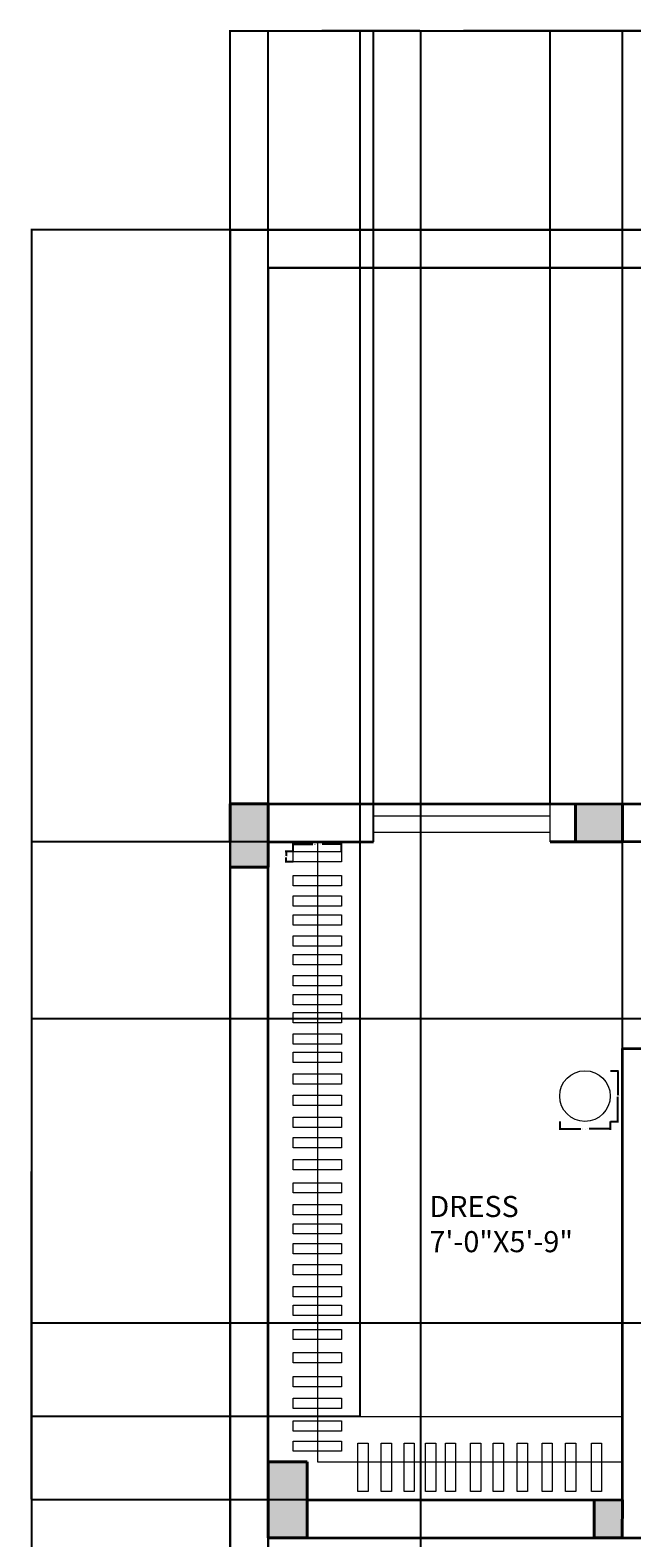
# Model space of a CAD drawing. Units: inches. Extents: x 1210 to 1836, y 84 to 1122.
# Tile 3 of 5: x 1210 to 1353, y 764 to 1122. Entities that reach past the tile are written whole.
import ezdxf

# ---------------------------------------------------------------- set-up
doc = ezdxf.new("R2010")
doc.units = ezdxf.units.IN
doc.header["$MEASUREMENT"] = 0
for name, color, linetype, lineweight in [('A-ANNO-DIMS', 2, 'Continuous', 18), ('A-AREA-IDEN', 7, 'Continuous', 25), ('A-COLS', 7, 'Continuous', 40), ('A-COLS-PATT', 6, 'Continuous', 13), ('A-FURN', 9, 'Continuous', 18), ('A-FURN-FIXD', 32, 'Continuous', 18), ('A-GLAZ', 4, 'Continuous', 18), ('A-WALL', 7, 'Continuous', 35), ('C-PROP', 32, 'Continuous', 30)]:
    doc.layers.add(name, color=color, linetype=linetype, lineweight=lineweight)
doc.styles.get("Standard").update_dxf_attribs({"font": 'arial.ttf'})
doc.dimstyles.get("Standard").update_dxf_attribs({"dimtxt": 0.18, "dimasz": 0.18, "dimexe": 0.18, "dimexo": 0.0625, "dimgap": 0.09, "dimtad": 0, "dimtih": 1, "dimtoh": 1, "dimdec": 4, "dimzin": 0, "dimdsep": 46, "dimtxsty": 'Standard', "dimcen": 0.09, "dimadec": 0, "dimazin": 0, "dimtfac": 1, "dimtdec": 4, "dimtofl": 0, "dimtmove": 0, "dimatfit": 3, "dimfxl": 1, "dimtolj": 1, "dimtzin": 0, "dimarcsym": 0})

# ---------------------------------------------------------------- blocks, each defined once
blk = doc.blocks.new('WARDROBE-HANGER')
for p, q in [((0, 0), (0, 2.42)), ((0, 2.42), (11.47, 2.42)), ((10.31, 0), (0, 0)), ((11.47, 0), (10.31, 0)), ((11.47, 2.42), (11.47, 0))]:
    blk.add_line(p, q)
blk = doc.blocks.new('STOOL-ROUND')
blk.add_circle((6, 6), 6)
blk = doc.blocks.new('*D12')
at = {"layer": 'A-ANNO-DIMS', "color": 0, "lineweight": -2, "transparency": 16777216}
for p, q in [((1272.27, 926.95), (1272.27, 928.79)), ((1272.45, 928.61), (1276.9, 928.61)), ((1283.55, 928.61), (1279.1, 928.61)), ((1283.73, 926.95), (1283.73, 928.79))]:
    blk.add_line(p, q, dxfattribs=at)
at = {"layer": 'A-ANNO-DIMS', "color": 0, "transparency": 16777216}
for points in [[(1272.45, 928.64), (1272.45, 928.58), (1272.27, 928.61)], [(1283.55, 928.64), (1283.55, 928.58), (1283.73, 928.61)]]:
    blk.add_solid(points, dxfattribs=at)
at = {"layer": 'Defpoints', "color": 0, "transparency": 16777216}
for p in [(1272.27, 926.89), (1283.73, 928.61), (1283.73, 926.89)]:
    blk.add_point(p, dxfattribs=at)
at = {"layer": 'A-ANNO-DIMS', "color": 0, "transparency": 16777216, "insert": (1278, 928.61), "char_height": 0.18, "attachment_point": 5}
blk.add_mtext('\\A1;HANGER 11 TYP.', dxfattribs=at)
blk = doc.blocks.new('*D13')
at = {"layer": 'A-ANNO-DIMS', "color": 0, "lineweight": -2, "transparency": 16777216}
for p, q in [((1272.2, 926.89), (1270.37, 926.89)), ((1270.55, 926.71), (1270.55, 925.85)), ((1272.2, 924.46), (1270.37, 924.46)), ((1270.55, 924.64), (1270.55, 925.49))]:
    blk.add_line(p, q, dxfattribs=at)
at = {"layer": 'A-ANNO-DIMS', "color": 0, "transparency": 16777216}
for points in [[(1270.52, 926.71), (1270.58, 926.71), (1270.55, 926.89)], [(1270.52, 924.64), (1270.58, 924.64), (1270.55, 924.46)]]:
    blk.add_solid(points, dxfattribs=at)
at = {"layer": 'Defpoints', "color": 0, "transparency": 16777216}
for p in [(1270.55, 926.89), (1272.27, 926.89), (1272.27, 924.46)]:
    blk.add_point(p, dxfattribs=at)
at = {"layer": 'A-ANNO-DIMS', "color": 0, "transparency": 16777216, "insert": (1270.55, 925.67), "char_height": 0.18, "attachment_point": 5}
blk.add_mtext('\\A1;2 TYP.', dxfattribs=at)
blk = doc.blocks.new('*D14')
at = {"layer": 'A-ANNO-DIMS', "color": 0, "lineweight": -2, "transparency": 16777216}
for p, q in [((1335.45, 862.86), (1335.45, 860.95)), ((1347.45, 862.86), (1347.45, 860.95)), ((1335.63, 861.13), (1340.46, 861.13)), ((1347.27, 861.13), (1342.44, 861.13))]:
    blk.add_line(p, q, dxfattribs=at)
at = {"layer": 'A-ANNO-DIMS', "color": 0, "transparency": 16777216}
for points in [[(1335.63, 861.16), (1335.63, 861.1), (1335.45, 861.13)], [(1347.27, 861.16), (1347.27, 861.1), (1347.45, 861.13)]]:
    blk.add_solid(points, dxfattribs=at)
at = {"layer": 'Defpoints', "color": 0, "transparency": 16777216}
for p in [(1335.45, 862.93), (1347.45, 862.93), (1347.45, 861.13)]:
    blk.add_point(p, dxfattribs=at)
at = {"layer": 'A-ANNO-DIMS', "color": 0, "transparency": 16777216, "insert": (1341.45, 861.13), "char_height": 0.18, "attachment_point": 5}
blk.add_mtext('\\A1;STOOL 12 TYP.', dxfattribs=at)
blk = doc.blocks.new('*D15')
at = {"layer": 'A-ANNO-DIMS', "color": 0, "lineweight": -2, "transparency": 16777216}
for p, q in [((1347.51, 874.92), (1349.43, 874.92)), ((1349.25, 874.74), (1349.25, 869.11)), ((1349.25, 863.11), (1349.25, 868.74)), ((1347.51, 862.93), (1349.43, 862.93))]:
    blk.add_line(p, q, dxfattribs=at)
at = {"layer": 'A-ANNO-DIMS', "color": 0, "transparency": 16777216}
for points in [[(1349.22, 874.74), (1349.28, 874.74), (1349.25, 874.92)], [(1349.22, 863.11), (1349.28, 863.11), (1349.25, 862.93)]]:
    blk.add_solid(points, dxfattribs=at)
at = {"layer": 'Defpoints', "color": 0, "transparency": 16777216}
for p in [(1347.45, 874.92), (1349.25, 874.92), (1347.45, 862.93)]:
    blk.add_point(p, dxfattribs=at)
at = {"layer": 'A-ANNO-DIMS', "color": 0, "transparency": 16777216, "insert": (1349.25, 868.92), "char_height": 0.18, "attachment_point": 5}
blk.add_mtext('\\A1;12 TYP.', dxfattribs=at)
blk = doc.blocks.new('*D22')
at = {"layer": 'A-ANNO-DIMS', "color": 0, "lineweight": -2, "transparency": 16777216}
for p, q in [((1257.32, 1074.28), (1257.32, 1121.57)), ((1257.5, 1121.39), (1522.55, 1121.39)), ((1788.14, 1121.39), (1523.1, 1121.39)), ((1788.32, 1074.28), (1788.32, 1121.57))]:
    blk.add_line(p, q, dxfattribs=at)
at = {"layer": 'A-ANNO-DIMS', "color": 0, "transparency": 16777216}
for points in [[(1257.5, 1121.42), (1257.5, 1121.36), (1257.32, 1121.39)], [(1788.14, 1121.42), (1788.14, 1121.36), (1788.32, 1121.39)]]:
    blk.add_solid(points, dxfattribs=at)
at = {"layer": 'Defpoints', "color": 0, "transparency": 16777216}
for p in [(1788.32, 1121.39), (1257.32, 1074.21), (1788.32, 1074.21)]:
    blk.add_point(p, dxfattribs=at)
at = {"layer": 'A-ANNO-DIMS', "color": 0, "transparency": 16777216, "insert": (1522.82, 1121.39), "char_height": 0.18, "attachment_point": 5}
blk.add_mtext('\\A1;531', dxfattribs=at)
blk = doc.blocks.new('*D23')
at = {"layer": 'A-ANNO-DIMS', "color": 0, "lineweight": -2, "transparency": 16777216}
for p, q in [((1257.26, 1074.21), (1209.97, 1074.21)), ((1210.15, 1074.03), (1210.15, 602.9)), ((1210.15, 131.39), (1210.15, 602.53)), ((1257.26, 131.21), (1209.97, 131.21))]:
    blk.add_line(p, q, dxfattribs=at)
at = {"layer": 'A-ANNO-DIMS', "color": 0, "transparency": 16777216}
for points in [[(1210.12, 1074.03), (1210.18, 1074.03), (1210.15, 1074.21)], [(1210.12, 131.39), (1210.18, 131.39), (1210.15, 131.21)]]:
    blk.add_solid(points, dxfattribs=at)
at = {"layer": 'Defpoints', "color": 0, "transparency": 16777216}
for p in [(1210.15, 1074.21), (1257.32, 1074.21), (1257.32, 131.21)]:
    blk.add_point(p, dxfattribs=at)
at = {"layer": 'A-ANNO-DIMS', "color": 0, "transparency": 16777216, "insert": (1210.15, 602.71), "char_height": 0.18, "attachment_point": 5}
blk.add_mtext('\\A1;943', dxfattribs=at)
blk = doc.blocks.new('*D38')
at = {"layer": 'A-ANNO-DIMS', "color": 0, "lineweight": -2, "transparency": 16777216}
for p, q in [((1266.26, 929.21), (1209.97, 929.21)), ((1210.15, 929.03), (1210.15, 851.4)), ((1210.15, 773.39), (1210.15, 851.03)), ((1266.26, 773.21), (1209.97, 773.21))]:
    blk.add_line(p, q, dxfattribs=at)
at = {"layer": 'A-ANNO-DIMS', "color": 0, "transparency": 16777216}
for points in [[(1210.12, 929.03), (1210.18, 929.03), (1210.15, 929.21)], [(1210.12, 773.39), (1210.18, 773.39), (1210.15, 773.21)]]:
    blk.add_solid(points, dxfattribs=at)
at = {"layer": 'Defpoints', "color": 0, "transparency": 16777216}
for p in [(1210.15, 929.21), (1266.32, 929.21), (1266.32, 773.21)]:
    blk.add_point(p, dxfattribs=at)
at = {"layer": 'A-ANNO-DIMS', "color": 0, "transparency": 16777216, "insert": (1210.15, 851.21), "char_height": 0.18, "attachment_point": 5}
blk.add_mtext('\\A1;156', dxfattribs=at)
blk = doc.blocks.new('*D40')
at = {"layer": 'A-ANNO-DIMS', "color": 0, "lineweight": -2, "transparency": 16777216}
for p, q in [((1288.13, 793.02), (1288.13, 1121.57)), ((1288.31, 1121.39), (1318.9, 1121.39)), ((1350.14, 1121.39), (1319.55, 1121.39)), ((1350.32, 793.02), (1350.32, 1121.57))]:
    blk.add_line(p, q, dxfattribs=at)
at = {"layer": 'A-ANNO-DIMS', "color": 0, "transparency": 16777216}
for points in [[(1288.31, 1121.42), (1288.31, 1121.36), (1288.13, 1121.39)], [(1350.14, 1121.42), (1350.14, 1121.36), (1350.32, 1121.39)]]:
    blk.add_solid(points, dxfattribs=at)
at = {"layer": 'Defpoints', "color": 0, "transparency": 16777216}
for p in [(1350.32, 1121.39), (1288.13, 792.95), (1350.32, 792.95)]:
    blk.add_point(p, dxfattribs=at)
at = {"layer": 'A-ANNO-DIMS', "color": 0, "transparency": 16777216, "insert": (1319.23, 1121.39), "char_height": 0.18, "attachment_point": 5}
blk.add_mtext('\\A1;62.2', dxfattribs=at)
blk = doc.blocks.new('*D41')
at = {"layer": 'A-ANNO-DIMS', "color": 0, "lineweight": -2, "transparency": 16777216}
for p, q in [((1288.07, 792.95), (1209.97, 792.95)), ((1210.15, 792.77), (1210.15, 783.27)), ((1210.15, 773.39), (1210.15, 782.9)), ((1275.46, 773.21), (1209.97, 773.21))]:
    blk.add_line(p, q, dxfattribs=at)
at = {"layer": 'A-ANNO-DIMS', "color": 0, "transparency": 16777216}
for points in [[(1210.12, 792.77), (1210.18, 792.77), (1210.15, 792.95)], [(1210.12, 773.39), (1210.18, 773.39), (1210.15, 773.21)]]:
    blk.add_solid(points, dxfattribs=at)
at = {"layer": 'Defpoints', "color": 0, "transparency": 16777216}
for p in [(1210.15, 792.95), (1288.13, 792.95), (1275.52, 773.21)]:
    blk.add_point(p, dxfattribs=at)
at = {"layer": 'A-ANNO-DIMS', "color": 0, "transparency": 16777216, "insert": (1210.15, 783.08), "char_height": 0.18, "attachment_point": 5}
blk.add_mtext('\\A1;19.74', dxfattribs=at)
blk = doc.blocks.new('*D45')
at = {"layer": 'A-ANNO-DIMS', "color": 0, "lineweight": -2, "transparency": 16777216}
for p, q in [((1449.78, 887.21), (1209.97, 887.21)), ((1210.15, 887.03), (1210.15, 851.34)), ((1210.15, 815.3), (1210.15, 850.98)), ((1449.78, 815.12), (1209.97, 815.12))]:
    blk.add_line(p, q, dxfattribs=at)
at = {"layer": 'A-ANNO-DIMS', "color": 0, "transparency": 16777216}
for points in [[(1210.12, 887.03), (1210.18, 887.03), (1210.15, 887.21)], [(1210.12, 815.3), (1210.18, 815.3), (1210.15, 815.12)]]:
    blk.add_solid(points, dxfattribs=at)
at = {"layer": 'Defpoints', "color": 0, "transparency": 16777216}
for p in [(1449.85, 887.21), (1210.15, 815.12), (1449.85, 815.12)]:
    blk.add_point(p, dxfattribs=at)
at = {"layer": 'A-ANNO-DIMS', "color": 0, "transparency": 16777216, "insert": (1210.15, 851.16), "char_height": 0.18, "attachment_point": 5}
blk.add_mtext('\\A1;72.1', dxfattribs=at)
blk = doc.blocks.new('*D49')
at = {"layer": 'A-ANNO-DIMS', "color": 0, "lineweight": -2, "transparency": 16777216}
for p, q in [((1266.32, 929.28), (1266.32, 1121.57)), ((1266.5, 1121.39), (1278.6, 1121.39)), ((1291.14, 1121.39), (1279.05, 1121.39)), ((1291.32, 929.28), (1291.32, 1121.57))]:
    blk.add_line(p, q, dxfattribs=at)
at = {"layer": 'A-ANNO-DIMS', "color": 0, "transparency": 16777216}
for points in [[(1266.5, 1121.42), (1266.5, 1121.36), (1266.32, 1121.39)], [(1291.14, 1121.42), (1291.14, 1121.36), (1291.32, 1121.39)]]:
    blk.add_solid(points, dxfattribs=at)
at = {"layer": 'Defpoints', "color": 0, "transparency": 16777216}
for p in [(1291.32, 1121.39), (1266.32, 929.21), (1291.32, 929.21)]:
    blk.add_point(p, dxfattribs=at)
at = {"layer": 'A-ANNO-DIMS', "color": 0, "transparency": 16777216, "insert": (1278.82, 1121.39), "char_height": 0.18, "attachment_point": 5}
blk.add_mtext('\\A1;25', dxfattribs=at)
blk = doc.blocks.new('*D50')
at = {"layer": 'A-ANNO-DIMS', "color": 0, "lineweight": -2, "transparency": 16777216}
for p, q in [((1291.32, 938.28), (1291.32, 1121.57)), ((1291.5, 1121.39), (1311.87, 1121.39)), ((1333.03, 1121.39), (1312.66, 1121.39)), ((1333.21, 938.28), (1333.21, 1121.57))]:
    blk.add_line(p, q, dxfattribs=at)
at = {"layer": 'A-ANNO-DIMS', "color": 0, "transparency": 16777216}
for points in [[(1291.5, 1121.42), (1291.5, 1121.36), (1291.32, 1121.39)], [(1333.03, 1121.42), (1333.03, 1121.36), (1333.21, 1121.39)]]:
    blk.add_solid(points, dxfattribs=at)
at = {"layer": 'Defpoints', "color": 0, "transparency": 16777216}
for p in [(1333.21, 1121.39), (1291.32, 938.21), (1333.21, 938.21)]:
    blk.add_point(p, dxfattribs=at)
at = {"layer": 'A-ANNO-DIMS', "color": 0, "transparency": 16777216, "insert": (1312.26, 1121.39), "char_height": 0.18, "attachment_point": 5}
blk.add_mtext('\\A1;41.88', dxfattribs=at)
blk = doc.blocks.new('*D51')
at = {"layer": 'A-ANNO-DIMS', "color": 0, "lineweight": -2, "transparency": 16777216}
for p, q in [((1333.21, 938.28), (1333.21, 1121.57)), ((1333.39, 1121.39), (1364.51, 1121.39)), ((1396.41, 1121.39), (1365.29, 1121.39)), ((1396.59, 938.28), (1396.59, 1121.57))]:
    blk.add_line(p, q, dxfattribs=at)
at = {"layer": 'A-ANNO-DIMS', "color": 0, "transparency": 16777216}
for points in [[(1333.39, 1121.42), (1333.39, 1121.36), (1333.21, 1121.39)], [(1396.41, 1121.42), (1396.41, 1121.36), (1396.59, 1121.39)]]:
    blk.add_solid(points, dxfattribs=at)
at = {"layer": 'Defpoints', "color": 0, "transparency": 16777216}
for p in [(1396.59, 1121.39), (1333.21, 938.21), (1396.59, 938.21)]:
    blk.add_point(p, dxfattribs=at)
at = {"layer": 'A-ANNO-DIMS', "color": 0, "transparency": 16777216, "insert": (1364.9, 1121.39), "char_height": 0.18, "attachment_point": 5}
blk.add_mtext('\\A1;63.39', dxfattribs=at)
blk = doc.blocks.new('*D72')
at = {"layer": 'A-ANNO-DIMS', "color": 0, "lineweight": -2, "transparency": 16777216}
for p, q in [((1257.32, 590.28), (1257.32, 1121.57)), ((1257.5, 1121.39), (1279.44, 1121.39)), ((1302.31, 1121.39), (1280.37, 1121.39)), ((1302.49, 590.28), (1302.49, 1121.57))]:
    blk.add_line(p, q, dxfattribs=at)
at = {"layer": 'A-ANNO-DIMS', "color": 0, "transparency": 16777216}
for points in [[(1257.5, 1121.42), (1257.5, 1121.36), (1257.32, 1121.39)], [(1302.31, 1121.42), (1302.31, 1121.36), (1302.49, 1121.39)]]:
    blk.add_solid(points, dxfattribs=at)
at = {"layer": 'Defpoints', "color": 0, "transparency": 16777216}
for p in [(1302.49, 1121.39), (1257.32, 590.21), (1302.49, 590.21)]:
    blk.add_point(p, dxfattribs=at)
at = {"layer": 'A-ANNO-DIMS', "color": 0, "transparency": 16777216, "insert": (1279.91, 1121.39), "char_height": 0.18, "attachment_point": 5}
blk.add_mtext('\\A1;45.165', dxfattribs=at)
blk = doc.blocks.new('*D73')
at = {"layer": 'A-ANNO-DIMS', "color": 0, "lineweight": -2, "transparency": 16777216}
for p, q in [((1302.49, 590.28), (1302.49, 1121.57)), ((1302.67, 1121.39), (1339.91, 1121.39)), ((1377.81, 1121.39), (1340.56, 1121.39)), ((1377.99, 590.28), (1377.99, 1121.57))]:
    blk.add_line(p, q, dxfattribs=at)
at = {"layer": 'A-ANNO-DIMS', "color": 0, "transparency": 16777216}
for points in [[(1302.67, 1121.42), (1302.67, 1121.36), (1302.49, 1121.39)], [(1377.81, 1121.42), (1377.81, 1121.36), (1377.99, 1121.39)]]:
    blk.add_solid(points, dxfattribs=at)
at = {"layer": 'Defpoints', "color": 0, "transparency": 16777216}
for p in [(1377.99, 1121.39), (1302.49, 590.21), (1377.99, 590.21)]:
    blk.add_point(p, dxfattribs=at)
at = {"layer": 'A-ANNO-DIMS', "color": 0, "transparency": 16777216, "insert": (1340.24, 1121.39), "char_height": 0.18, "attachment_point": 5}
blk.add_mtext('\\A1;75.5', dxfattribs=at)

msp = doc.modelspace()

# ---------------------------------------------------------------- hatches: boundary and pattern name
at = {"layer": 'A-COLS-PATT'}
h = msp.add_hatch(color=256, dxfattribs=at)
h.dxf.hatch_style = 1
h.paths.add_polyline_path([(1266.3239, 938.214), (1257.3239, 938.214), (1257.3239, 929.4573), (1257.3239, 923.2025), (1266.3239, 923.2025)])
h.paths.add_polyline_path([(1350.3239, 929.214), (1350.3239, 938.214), (1339.1886, 938.214), (1339.1886, 929.214)])
h.paths.add_polyline_path([(1559.1961, 929.214), (1559.1961, 938.214), (1542.8626, 938.214), (1542.8626, 929.214), (1543.3239, 929.214)])
h.paths.add_polyline_path([(1771.5139, 938.214), (1771.5139, 929.214), (1788.3239, 929.214), (1788.3239, 938.214)])
h.paths.add_polyline_path([(1788.3239, 764.214), (1788.3239, 773.214), (1775.2119, 773.214), (1775.2119, 764.214)])
h.paths.add_polyline_path([(1552.3239, 764.214), (1552.3239, 773.214), (1543.3239, 773.214), (1535.8494, 773.197), (1535.8494, 764.214)])
h.paths.add_polyline_path([(1275.5217, 782.2138), (1272.7843, 782.2138), (1266.3239, 782.2138), (1266.3239, 764.214), (1275.5217, 764.214)])
h.paths.add_polyline_path([(1350.2372, 764.214), (1350.3239, 773.214), (1343.6352, 773.214), (1343.6352, 764.214)])
h.paths.add_polyline_path([(1257.3239, 570.3846), (1266.3239, 570.3846), (1266.3239, 590.214), (1257.3239, 590.214)])
h.paths.add_polyline_path([(1450.8239, 572.5809), (1459.8239, 572.5809), (1459.8239, 590.214), (1458.3239, 590.214), (1450.8239, 590.214)])
h.paths.add_polyline_path([(1531.8239, 572.5809), (1540.8239, 572.5809), (1540.8239, 590.214), (1531.8239, 590.214)])
h.paths.add_polyline_path([(1450.8239, 392.214), (1459.8239, 392.214), (1459.8239, 401.214), (1459.8239, 408.7866), (1450.8239, 408.7866)])
h.paths.add_polyline_path([(1531.8239, 392.214), (1540.8239, 392.214), (1540.8239, 401.214), (1540.8239, 408.7866), (1531.8239, 408.7866)])
h.paths.add_polyline_path([(1682.9725, 401.214), (1682.9725, 392.214), (1698.3239, 392.214), (1698.3239, 401.214), (1693.8239, 401.214)])
h.paths.add_polyline_path([(1774.197, 350.714), (1779.3239, 350.714), (1788.3239, 350.714), (1788.3239, 359.714), (1779.3239, 359.714), (1774.197, 359.714)])
h.paths.add_polyline_path([(1779.3239, 590.214), (1775.4485, 590.214), (1775.4485, 581.214), (1779.3239, 581.214), (1788.3239, 581.214), (1788.3239, 590.214)])

# ---------------------------------------------------------------- linework, layer by layer
at = {"layer": 'A-COLS'}
for p, q in [((1266.3239, 938.214), (1257.3239, 938.214)), ((1257.3239, 938.214), (1257.3239, 929.4573)), ((1266.3239, 929.4573), (1266.3239, 938.214)), ((1266.3239, 938.214), (1266.3239, 923.2025)), ((1339.1886, 938.214), (1339.1886, 929.214)), ((1350.3239, 929.214), (1350.3239, 938.214)), ((1339.1886, 929.214), (1350.3239, 929.214)), ((1266.3239, 923.2025), (1257.3239, 923.2025)), ((1266.3239, 764.214), (1266.3239, 782.2138)), ((1266.3239, 782.2138), (1272.7843, 782.2138)), ((1272.7843, 782.2138), (1275.5217, 782.2138)), ((1275.5217, 782.2138), (1275.5217, 764.214)), ((1275.5217, 764.214), (1266.3239, 764.214))]:
    msp.add_line(p, q, dxfattribs=at)
msp.add_lwpolyline([(1350.3239, 773.214), (1350.2372, 764.214), (1343.6352, 764.214), (1343.6352, 773.214)], dxfattribs=at)
at = {"layer": 'A-FURN-FIXD'}
for p, q in [((1278.0003, 929.214), (1278.0003, 782.2138)), ((1288.1277, 929.214), (1288.1277, 792.9531)), ((1288.1277, 792.9531), (1350.3239, 792.9531)), ((1278.0003, 782.2138), (1350.3239, 782.2138))]:
    msp.add_line(p, q, dxfattribs=at)
at = {"layer": 'A-GLAZ'}
for p, q in [((1291.3243, 938.214), (1291.3243, 929.214)), ((1333.2056, 929.214), (1333.2056, 938.214)), ((1333.2056, 935.2386), (1291.3243, 935.2386)), ((1333.2056, 931.4993), (1333.2056, 935.2386)), ((1291.3243, 931.4993), (1333.2056, 931.4993))]:
    msp.add_line(p, q, dxfattribs=at)
at = {"layer": 'A-WALL'}
for p, q in [((1266.3239, 938.214), (1673.9914, 938.214)), ((1333.2056, 938.214), (1339.1886, 938.214)), ((1350.3239, 938.214), (1396.5935, 938.214)), ((1266.3239, 929.214), (1291.3243, 929.214)), ((1266.3239, 773.214), (1266.3239, 929.214)), ((1333.2056, 929.214), (1350.3239, 929.214)), ((1354.8239, 929.214), (1333.2056, 929.214)), ((1350.3239, 773.214), (1350.3239, 880.2123)), ((1350.3239, 880.2123), (1354.8239, 880.2123)), ((1275.5217, 773.214), (1350.3239, 773.214)), ((1266.3239, 764.214), (1419.0081, 764.214))]:
    msp.add_line(p, q, dxfattribs=at)
at = {"layer": 'C-PROP'}
for p, q in [((1257.3239, 131.214), (1257.3239, 1074.214)), ((1257.3239, 1074.214), (1788.3239, 1074.214)), ((1266.3239, 1065.214), (1779.3239, 1065.214)), ((1266.3239, 938.214), (1266.3239, 1065.214)), ((1266.3239, 140.214), (1266.3239, 764.214))]:
    msp.add_line(p, q, dxfattribs=at)

# ---------------------------------------------------------------- block references
at = {"layer": 'A-FURN'}
msp.add_blockref('STOOL-ROUND', (1335.45, 862.926), dxfattribs=at)
at = {"layer": 'A-FURN-FIXD'}
for p in [(1272.267, 924.461), (1272.267, 918.7888), (1272.267, 913.9748), (1272.267, 909.4525), (1272.267, 904.4925), (1272.267, 900.0432), (1272.267, 895.0675), (1272.267, 890.5452), (1272.267, 886.2931), (1272.267, 881.2602), (1272.267, 876.8838), (1272.267, 871.778), (1272.267, 866.7286), (1272.267, 861.4779), (1272.267, 856.694), (1272.267, 851.4433), (1272.267, 845.9593), (1272.267, 840.7842), (1272.267, 836.2336), (1272.267, 831.5663), (1272.267, 826.549), (1272.267, 821.3667), (1272.267, 816.9328), (1272.267, 811.2154), (1272.267, 805.7313), (1272.267, 800.0139), (1272.267, 794.8799), (1272.267, 789.5126), (1272.267, 784.7286)]:
    msp.add_blockref('WARDROBE-HANGER', p, dxfattribs=at)
for p, rotation in [((1290.0135, 775.2221), 89.99999999999696), ((1295.5557, 775.2221), 89.99999999999883), ((1300.9642, 775.2221), 89.99999999999696), ((1306.0803, 775.2221), 89.99999999999883), ((1310.7578, 775.2221), 89.99999999999883), ((1316.751, 775.2221), 89.99999999999883), ((1322.0863, 775.2221), 89.99999999999696), ((1327.7871, 775.2221), 89.99999999999696), ((1333.7071, 775.2221), 89.99999999999883), ((1339.2618, 775.2221), 90.00000000000072), ((1345.4011, 775.2221), 89.99999999999883)]:
    msp.add_blockref('WARDROBE-HANGER', p, dxfattribs=dict(at, rotation=rotation))

# ---------------------------------------------------------------- texts
at = {"layer": 'A-AREA-IDEN', "insert": (1304.5589, 845.2509), "char_height": 5, "attachment_point": 1}
msp.add_mtext_dynamic_manual_height_columns('{DRESS\\P7\'-0"X5\'-9"}', width=293.611423, gutter_width=1, heights=[0], dxfattribs=at)

# ---------------------------------------------------------------- dimensions: what is measured, and where the dimension line sits
at = {"layer": 'A-ANNO-DIMS'}
for base, p1, p2, override, picture, middle in [((1788.3239, 1121.389), (1257.3239, 1074.214), (1788.3239, 1074.214), {"dimdec": 0, "dimlfac": 1, "dimrnd": 0, "dimzin": 0, "dimdsep": 46, "dimlunit": 2}, '*D22', (1522.8239, 1121.389)), ((1302.4894, 1121.38901), (1257.32392, 590.21401), (1302.4894, 590.21401), {"dimdec": 3, "dimlfac": 1, "dimrnd": 0, "dimzin": 0, "dimdsep": 46, "dimlunit": 2}, '*D72', (1279.90666, 1121.38901)), ((1291.3243, 1121.389), (1266.3239, 929.214), (1291.3243, 929.214), {"dimdec": 0, "dimlfac": 1, "dimrnd": 0, "dimzin": 0, "dimdsep": 46, "dimlunit": 2}, '*D49', (1278.8241, 1121.389)), ((1350.3239, 1121.389), (1288.1277, 792.9531), (1350.3239, 792.9531), {"dimdec": 1, "dimlfac": 1, "dimrnd": 0, "dimzin": 0, "dimdsep": 46, "dimlunit": 2}, '*D40', (1319.2258, 1121.389)), ((1333.2056, 1121.389), (1291.3243, 938.214), (1333.2056, 938.214), {"dimdec": 2, "dimlfac": 1, "dimrnd": 0, "dimzin": 0, "dimdsep": 46, "dimlunit": 2}, '*D50', (1312.2649, 1121.389)), ((1377.9853, 1121.389), (1302.4894, 590.214), (1377.9853, 590.214), {"dimdec": 1, "dimlfac": 1, "dimrnd": 0, "dimzin": 0, "dimdsep": 46, "dimlunit": 2}, '*D73', (1340.2374, 1121.389)), ((1396.5935, 1121.389), (1333.2056, 938.214), (1396.5935, 938.214), {"dimdec": 2, "dimlfac": 1, "dimrnd": 0, "dimzin": 0, "dimdsep": 46, "dimlunit": 2}, '*D51', (1364.8996, 1121.389))]:
    dim = msp.add_linear_dim(base=base, p1=p1, p2=p2, dimstyle='Standard', override=override, dxfattribs=at)
    dim.commit()
    dim.dimension.update_dxf_attribs({"geometry": picture, "text_midpoint": middle})
for base, p1, p2, override, picture, middle in [((1210.1489, 1074.214), (1257.3239, 131.214), (1257.3239, 1074.214), {"dimdec": 0, "dimlfac": 1, "dimrnd": 0, "dimzin": 0, "dimdsep": 46, "dimlunit": 2}, '*D23', (1210.1489, 602.714)), ((1210.1489, 929.214), (1266.3239, 773.214), (1266.3239, 929.214), {"dimdec": 0, "dimlfac": 1, "dimrnd": 0, "dimzin": 0, "dimdsep": 46, "dimlunit": 2}, '*D38', (1210.1489, 851.214)), ((1210.1489, 815.1167), (1449.8451, 887.2124), (1449.8451, 815.1167), {"dimdec": 1, "dimlfac": 1, "dimrnd": 0, "dimzin": 0, "dimdsep": 46, "dimlunit": 2}, '*D45', (1210.1489, 851.1646)), ((1210.1489, 792.9531), (1275.5217, 773.214), (1288.1277, 792.9531), {"dimdec": 2, "dimlfac": 1, "dimrnd": 0, "dimzin": 0, "dimdsep": 46, "dimlunit": 2}, '*D41', (1210.1489, 783.0836))]:
    dim = msp.add_linear_dim(base=base, p1=p1, p2=p2, angle=90, dimstyle='Standard', override=override, dxfattribs=at)
    dim.commit()
    dim.dimension.update_dxf_attribs({"geometry": picture, "text_midpoint": middle})
for base, p1, p2, picture, middle in [((1270.5475, 926.8853), (1272.2673, 924.4611), (1272.2673, 926.8853), '*D13', (1270.5475, 925.6732)), ((1349.2454, 874.9229), (1347.4459, 862.9265), (1347.4459, 874.9229), '*D15', (1349.2454, 868.9247))]:
    dim = msp.add_linear_dim(base=base, p1=p1, p2=p2, angle=90, text='<> TYP.', dimstyle='Standard', override={"dimdec": 0, "dimlfac": 1, "dimrnd": 0, "dimzin": 0, "dimdsep": 46, "dimlunit": 2}, dxfattribs=at)
    dim.commit()
    dim.dimension.update_dxf_attribs({"geometry": picture, "text_midpoint": middle})
for base, p1, p2, text, picture, middle in [((1283.7332, 928.6052), (1272.2673, 926.8853), (1283.7332, 926.8853), 'HANGER <> TYP.', '*D12', (1278.0003, 928.6052)), ((1347.4459, 861.127), (1335.4495, 862.9265), (1347.4459, 862.9265), 'STOOL <> TYP.', '*D14', (1341.4477, 861.127))]:
    dim = msp.add_linear_dim(base=base, p1=p1, p2=p2, text=text, dimstyle='Standard', override={"dimdec": 0, "dimlfac": 1, "dimrnd": 0, "dimzin": 0, "dimdsep": 46, "dimlunit": 2}, dxfattribs=at)
    dim.commit()
    dim.dimension.update_dxf_attribs({"geometry": picture, "text_midpoint": middle})

doc.saveas('drawing.dxf')
